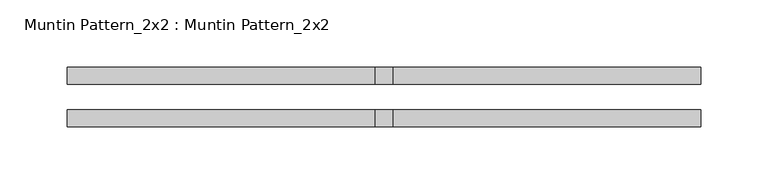
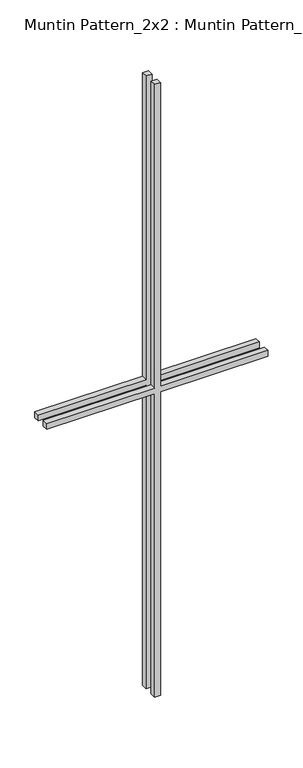
"""IFC4 building model written with IfcOpenShell, lengths in millimetres: proxy geometry, Muntin Pattern_2x2 : Muntin Pattern_2x2."""

from ifc_helpers import new_model, si_unit, frame, origin, place, context, project, spatial, polyline, outline, extrude, source, transform, mapped, element, save


def muntin_pattern_2x2_muntin_pattern_2x2_a30a3345(model_context):
    return source(origin(), model_context, "Body", "SweptSolid", [
        extrude(outline(polyline([(698.5, -6.35), (698.5, -236.5375), (685.8, -236.5375), (685.8, -6.35), (0.0, -6.35), (0.0, 6.35), (685.8, 6.35), (685.8, 236.5375), (698.5, 236.5375), (698.5, 6.35), (1384.3, 6.35), (1384.3, -6.35), (698.5, -6.35)])), frame((0.0, -22.225, 0.0), z_axis=(0.0, 1.0, 0.0), x_axis=(0.0, 0.0, 1.0)), (0.0, 0.0, 1.0), 12.7),
        extrude(outline(polyline([(698.5, -6.35), (698.5, -236.5375), (685.8, -236.5375), (685.8, -6.35), (0.0, -6.35), (0.0, 6.35), (685.8, 6.35), (685.8, 236.5375), (698.5, 236.5375), (698.5, 6.35), (1384.3, 6.35), (1384.3, -6.35), (698.5, -6.35)])), frame((0.0, 9.525, 0.0), z_axis=(0.0, 1.0, 0.0), x_axis=(0.0, 0.0, 1.0)), (0.0, 0.0, 1.0), 12.7),
    ])


if __name__ == "__main__":
    model = new_model("IFC4")
    model_context = context("Model", 3, world=origin())
    ifc_project = project(units=[si_unit("LENGTHUNIT", "METRE", prefix="MILLI")], contexts=[model_context])
    site = spatial("IfcSite", under=ifc_project)
    building = spatial("IfcBuilding", under=site)
    placement = place(None, origin())
    muntin_pattern_2x2_muntin_pattern_2x2_shape = muntin_pattern_2x2_muntin_pattern_2x2_a30a3345(model_context)
    element("IfcBuildingElementProxy", 1, Name="Muntin Pattern_2x2 : Muntin Pattern_2x2", ObjectType="Muntin Pattern_2x2 : Muntin Pattern_2x2", at=placement, inside=building, context=model_context, shape_type="MappedRepresentation", body=[
        mapped(muntin_pattern_2x2_muntin_pattern_2x2_shape, transform((0.0, 0.0, 0.0), x_axis=(1.0, 0.0, 0.0), y_axis=(0.0, 1.0, 0.0), z_axis=(0.0, 0.0, 1.0))),
    ])
    save(model, "model.ifc")

# Revit data of these elements
# Type "Muntin Pattern_2x2 : Muntin Pattern_2x2"
#   Width [instance default] = 4' - 0"
#   Thickness = 0' - 0 1/2"
#   Height [instance default] = 4' - 0"
#   Distance = 0' - 0 3/4"
#   Interior Material [instance default] = none
#   Exterior Material [instance default] = none
#   Default Elevation = 0
# Element 1 (IfcBuildingElementProxy, "Muntin Pattern_2x2 : Muntin Pattern_2x2")
#   Width = 1' - 6 5/8"
#   Height = 4' - 6 1/2"
#   Interior Material = Wood - Stained
#   Exterior Material = Clad - White
#   Materials on its faces: "Clad - White", "Wood - Stained"
# Materials
#   "Clad - White": class "Wood", colour RGB 245 245 243, transparency 0, Cost = 0
#   "Wood - Stained": class "Wood", colour RGB 173 132 96, transparency 0, Cost = 0
